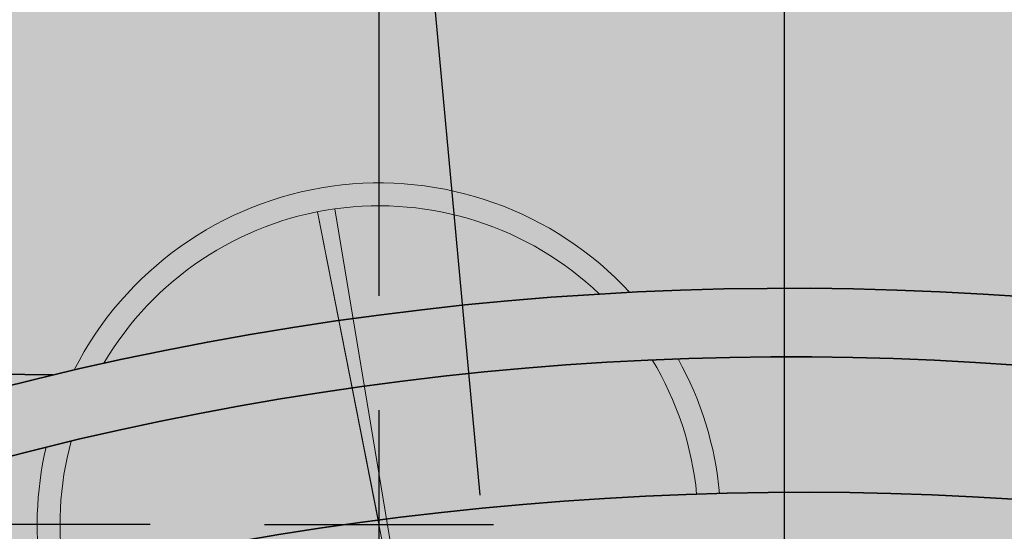
# Model space of a CAD drawing. Units: millimetres. Extents: x 130 to 1021, y 147 to 699.
# Tile 22 of 40: x 399 to 442, y 501 to 523. Entities that reach past the tile are written whole.
import ezdxf

# ---------------------------------------------------------------- set-up
doc = ezdxf.new("R2010")
doc.units = ezdxf.units.MM
doc.header["$MEASUREMENT"] = 0
for name, color, linetype, lineweight in [('A-ANNO-DIMS', 2, 'Continuous', 18), ('A-ELEV', 7, 'Continuous', 35), ('A-ELEV-PATT', 9, 'Continuous', 13), ('A-ELEV-RAIL', 6, 'Continuous', 18)]:
    doc.layers.add(name, color=color, linetype=linetype, lineweight=lineweight)
doc.styles.get("Standard").update_dxf_attribs({"font": 'arial.ttf'})
doc.dimstyles.get("Standard").update_dxf_attribs({"dimtxt": 20, "dimasz": 10, "dimexe": 10, "dimexo": 10, "dimgap": 5, "dimtad": 0, "dimtih": 1, "dimtoh": 1, "dimdec": 0, "dimzin": 0, "dimdsep": 46, "dimtxsty": 'Standard', "dimcen": 5, "dimadec": 0, "dimazin": 0, "dimtfac": 1, "dimtdec": 0, "dimtofl": 0, "dimtmove": 0, "dimatfit": 3, "dimfxl": 1, "dimtolj": 1, "dimtzin": 0, "dimarcsym": 0})

# ---------------------------------------------------------------- blocks, each defined once
blk = doc.blocks.new('*D11')
at = {"layer": 'A-ANNO-DIMS', "color": 0, "lineweight": -2, "transparency": 16777216}
for p, q in [((737.374, 648.699), (737.374, 149.739)), ((299.374, 566.947), (299.374, 149.739)), ((309.374, 159.739), (490.857, 159.739)), ((727.374, 159.739), (545.891, 159.739))]:
    blk.add_line(p, q, dxfattribs=at)
at = {"layer": 'A-ANNO-DIMS', "color": 0, "transparency": 16777216}
for points in [[(309.374, 161.406), (309.374, 158.073), (299.374, 159.739)], [(727.374, 161.406), (727.374, 158.073), (737.374, 159.739)]]:
    blk.add_solid(points, dxfattribs=at)
at = {"layer": 'Defpoints', "color": 0, "transparency": 16777216}
for p in [(737.374, 658.699), (299.374, 576.947), (737.374, 159.739)]:
    blk.add_point(p, dxfattribs=at)
at = {"layer": 'A-ANNO-DIMS', "color": 0, "transparency": 16777216, "insert": (518.374, 159.739), "char_height": 20, "attachment_point": 5}
blk.add_mtext('\\A1;438', dxfattribs=at)
blk = doc.blocks.new('*D12')
at = {"layer": 'A-ANNO-DIMS', "color": 0, "lineweight": -2, "transparency": 16777216}
for p, q in [((477.374, 661.947), (265.074, 661.947)), ((275.074, 651.947), (275.074, 438.205)), ((275.074, 194.039), (275.074, 407.782)), ((357.163, 184.039), (265.074, 184.039))]:
    blk.add_line(p, q, dxfattribs=at)
at = {"layer": 'A-ANNO-DIMS', "color": 0, "transparency": 16777216}
for points in [[(273.407, 651.947), (276.74, 651.947), (275.074, 661.947)], [(273.407, 194.039), (276.74, 194.039), (275.074, 184.039)]]:
    blk.add_solid(points, dxfattribs=at)
at = {"layer": 'Defpoints', "color": 0, "transparency": 16777216}
for p in [(275.074, 661.947), (487.374, 661.947), (367.163, 184.039)]:
    blk.add_point(p, dxfattribs=at)
at = {"layer": 'A-ANNO-DIMS', "color": 0, "transparency": 16777216, "insert": (275.074, 422.993), "char_height": 20, "attachment_point": 5}
blk.add_mtext('\\A1;477.9', dxfattribs=at)
blk = doc.blocks.new('*D15')
at = {"layer": 'A-ANNO-DIMS', "color": 0, "lineweight": -2, "transparency": 16777216}
for p, q in [((327.374, 579.884), (327.374, 696.247)), ((357.941, 411.947), (357.941, 696.247)), ((337.374, 686.247), (347.941, 686.247)), ((357.941, 686.247), (367.941, 686.247))]:
    blk.add_line(p, q, dxfattribs=at)
at = {"layer": 'A-ANNO-DIMS', "color": 0, "transparency": 16777216}
for points in [[(337.374, 687.914), (337.374, 684.581), (327.374, 686.247)], [(347.941, 687.914), (347.941, 684.581), (357.941, 686.247)]]:
    blk.add_solid(points, dxfattribs=at)
at = {"layer": 'Defpoints', "color": 0, "transparency": 16777216}
for p in [(357.941, 686.247), (327.374, 569.884), (357.941, 401.947)]:
    blk.add_point(p, dxfattribs=at)
at = {"layer": 'A-ANNO-DIMS', "color": 0, "transparency": 16777216, "insert": (406.679, 686.247), "char_height": 20, "attachment_point": 5}
blk.add_mtext('\\A1;30.57', dxfattribs=at)
blk = doc.blocks.new('*D16')
at = {"layer": 'A-ANNO-DIMS', "color": 0, "lineweight": -2, "transparency": 16777216}
for p, q in [((357.941, 411.947), (357.941, 696.247)), ((363.922, 579.884), (363.922, 696.247)), ((347.941, 686.247), (337.941, 686.247)), ((373.922, 686.247), (383.922, 686.247))]:
    blk.add_line(p, q, dxfattribs=at)
at = {"layer": 'A-ANNO-DIMS', "color": 0, "transparency": 16777216}
for points in [[(347.941, 687.914), (347.941, 684.581), (357.941, 686.247)], [(373.922, 687.914), (373.922, 684.581), (363.922, 686.247)]]:
    blk.add_solid(points, dxfattribs=at)
at = {"layer": 'Defpoints', "color": 0, "transparency": 16777216}
for p in [(363.922, 686.247), (363.922, 569.884), (357.941, 401.947)]:
    blk.add_point(p, dxfattribs=at)
at = {"layer": 'A-ANNO-DIMS', "color": 0, "transparency": 16777216, "insert": (420.737, 686.247), "char_height": 20, "attachment_point": 5}
blk.add_mtext('\\A1;5.981', dxfattribs=at)
blk = doc.blocks.new('*D17')
at = {"layer": 'A-ANNO-DIMS', "color": 0, "lineweight": -2, "transparency": 16777216}
for p, q in [((363.922, 579.884), (363.922, 696.247)), ((375.85, 490.216), (375.85, 696.247)), ((353.922, 686.247), (343.922, 686.247)), ((385.85, 686.247), (395.85, 686.247))]:
    blk.add_line(p, q, dxfattribs=at)
at = {"layer": 'A-ANNO-DIMS', "color": 0, "transparency": 16777216}
for points in [[(353.922, 687.914), (353.922, 684.581), (363.922, 686.247)], [(385.85, 687.914), (385.85, 684.581), (375.85, 686.247)]]:
    blk.add_solid(points, dxfattribs=at)
at = {"layer": 'Defpoints', "color": 0, "transparency": 16777216}
for p in [(375.85, 686.247), (363.922, 569.884), (375.85, 480.216)]:
    blk.add_point(p, dxfattribs=at)
at = {"layer": 'A-ANNO-DIMS', "color": 0, "transparency": 16777216, "insert": (441.444, 686.247), "char_height": 20, "attachment_point": 5}
blk.add_mtext('\\A1;11.928', dxfattribs=at)
blk = doc.blocks.new('*D18')
at = {"layer": 'A-ANNO-DIMS', "color": 0, "lineweight": -2, "transparency": 16777216}
for p, q in [((375.85, 490.216), (375.85, 696.247)), ((382.374, 388.947), (382.374, 696.247)), ((365.85, 686.247), (355.85, 686.247)), ((392.374, 686.247), (402.374, 686.247))]:
    blk.add_line(p, q, dxfattribs=at)
at = {"layer": 'A-ANNO-DIMS', "color": 0, "transparency": 16777216}
for points in [[(365.85, 687.914), (365.85, 684.581), (375.85, 686.247)], [(392.374, 687.914), (392.374, 684.581), (382.374, 686.247)]]:
    blk.add_solid(points, dxfattribs=at)
at = {"layer": 'Defpoints', "color": 0, "transparency": 16777216}
for p in [(382.374, 686.247), (375.85, 480.216), (382.374, 378.947)]:
    blk.add_point(p, dxfattribs=at)
at = {"layer": 'A-ANNO-DIMS', "color": 0, "transparency": 16777216, "insert": (441.132, 686.247), "char_height": 20, "attachment_point": 5}
blk.add_mtext('\\A1;6.524', dxfattribs=at)
blk = doc.blocks.new('*D19')
at = {"layer": 'A-ANNO-DIMS', "color": 0, "lineweight": -2, "transparency": 16777216}
for p, q in [((382.374, 388.947), (382.374, 696.247)), ((414.652, 510.881), (414.652, 696.247)), ((392.374, 686.247), (404.652, 686.247)), ((414.652, 686.247), (424.652, 686.247))]:
    blk.add_line(p, q, dxfattribs=at)
at = {"layer": 'A-ANNO-DIMS', "color": 0, "transparency": 16777216}
for points in [[(392.374, 687.914), (392.374, 684.581), (382.374, 686.247)], [(404.652, 687.914), (404.652, 684.581), (414.652, 686.247)]]:
    blk.add_solid(points, dxfattribs=at)
at = {"layer": 'Defpoints', "color": 0, "transparency": 16777216}
for p in [(414.652, 686.247), (414.652, 500.881), (382.374, 378.947)]:
    blk.add_point(p, dxfattribs=at)
at = {"layer": 'A-ANNO-DIMS', "color": 0, "transparency": 16777216, "insert": (463.411, 686.247), "char_height": 20, "attachment_point": 5}
blk.add_mtext('\\A1;32.28', dxfattribs=at)
blk = doc.blocks.new('*D20')
at = {"layer": 'A-ANNO-DIMS', "color": 0, "lineweight": -2, "transparency": 16777216}
for p, q in [((414.652, 510.881), (414.652, 696.247)), ((432.374, 388.947), (432.374, 696.247)), ((404.652, 686.247), (394.652, 686.247)), ((442.374, 686.247), (452.374, 686.247))]:
    blk.add_line(p, q, dxfattribs=at)
at = {"layer": 'A-ANNO-DIMS', "color": 0, "transparency": 16777216}
for points in [[(404.652, 687.914), (404.652, 684.581), (414.652, 686.247)], [(442.374, 687.914), (442.374, 684.581), (432.374, 686.247)]]:
    blk.add_solid(points, dxfattribs=at)
at = {"layer": 'Defpoints', "color": 0, "transparency": 16777216}
for p in [(432.374, 686.247), (414.652, 500.881), (432.374, 378.947)]:
    blk.add_point(p, dxfattribs=at)
at = {"layer": 'A-ANNO-DIMS', "color": 0, "transparency": 16777216, "insert": (490.075, 686.247), "char_height": 20, "attachment_point": 5}
blk.add_mtext('\\A1;17.72', dxfattribs=at)
blk = doc.blocks.new('*D21')
at = {"layer": 'A-ANNO-DIMS', "color": 0, "lineweight": -2, "transparency": 16777216}
for p, q in [((432.374, 388.947), (432.374, 696.247)), ((447.374, 656.947), (447.374, 696.247)), ((422.374, 686.247), (412.374, 686.247)), ((457.374, 686.247), (467.374, 686.247))]:
    blk.add_line(p, q, dxfattribs=at)
at = {"layer": 'A-ANNO-DIMS', "color": 0, "transparency": 16777216}
for points in [[(422.374, 687.914), (422.374, 684.581), (432.374, 686.247)], [(457.374, 687.914), (457.374, 684.581), (447.374, 686.247)]]:
    blk.add_solid(points, dxfattribs=at)
at = {"layer": 'Defpoints', "color": 0, "transparency": 16777216}
for p in [(447.374, 686.247), (447.374, 646.947), (432.374, 378.947)]:
    blk.add_point(p, dxfattribs=at)
at = {"layer": 'A-ANNO-DIMS', "color": 0, "transparency": 16777216, "insert": (485.832, 686.247), "char_height": 20, "attachment_point": 5}
blk.add_mtext('\\A1;15', dxfattribs=at)
blk = doc.blocks.new('*D22')
at = {"layer": 'A-ANNO-DIMS', "color": 0, "lineweight": -2, "transparency": 16777216}
for p, q in [((447.374, 656.947), (447.374, 696.247)), ((466.767, 403.947), (466.767, 696.247)), ((437.374, 686.247), (427.374, 686.247)), ((476.767, 686.247), (486.767, 686.247))]:
    blk.add_line(p, q, dxfattribs=at)
at = {"layer": 'A-ANNO-DIMS', "color": 0, "transparency": 16777216}
for points in [[(437.374, 687.914), (437.374, 684.581), (447.374, 686.247)], [(476.767, 687.914), (476.767, 684.581), (466.767, 686.247)]]:
    blk.add_solid(points, dxfattribs=at)
at = {"layer": 'Defpoints', "color": 0, "transparency": 16777216}
for p in [(466.767, 686.247), (447.374, 646.947), (466.767, 393.947)]:
    blk.add_point(p, dxfattribs=at)
at = {"layer": 'A-ANNO-DIMS', "color": 0, "transparency": 16777216, "insert": (532.34, 686.247), "char_height": 20, "attachment_point": 5}
blk.add_mtext('\\A1;19.393', dxfattribs=at)
blk = doc.blocks.new('*D43')
at = {"layer": 'A-ANNO-DIMS', "color": 0, "lineweight": -2, "transparency": 16777216}
for p, q in [((275.074, 510.881), (275.074, 520.881)), ((275.074, 520.881), (285.074, 520.881)), ((404.652, 500.881), (265.074, 500.881)), ((317.374, 480.95), (265.074, 480.95)), ((275.074, 470.95), (275.074, 460.95))]:
    blk.add_line(p, q, dxfattribs=at)
at = {"layer": 'A-ANNO-DIMS', "color": 0, "transparency": 16777216}
for points in [[(273.407, 510.881), (276.74, 510.881), (275.074, 500.881)], [(273.407, 470.95), (276.74, 470.95), (275.074, 480.95)]]:
    blk.add_solid(points, dxfattribs=at)
at = {"layer": 'Defpoints', "color": 0, "transparency": 16777216}
for p in [(275.074, 500.881), (414.652, 500.881), (327.374, 480.95)]:
    blk.add_point(p, dxfattribs=at)
at = {"layer": 'A-ANNO-DIMS', "color": 0, "transparency": 16777216, "insert": (322.877, 520.881), "char_height": 20, "attachment_point": 5}
blk.add_mtext('\\A1;19.93', dxfattribs=at)
blk = doc.blocks.new('*D44')
at = {"layer": 'A-ANNO-DIMS', "color": 0, "lineweight": -2, "transparency": 16777216}
for p, q in [((317.374, 569.884), (265.074, 569.884)), ((275.074, 559.884), (275.074, 550.594)), ((275.074, 510.881), (275.074, 520.171)), ((404.652, 500.881), (265.074, 500.881))]:
    blk.add_line(p, q, dxfattribs=at)
at = {"layer": 'A-ANNO-DIMS', "color": 0, "transparency": 16777216}
for points in [[(273.407, 559.884), (276.74, 559.884), (275.074, 569.884)], [(273.407, 510.881), (276.74, 510.881), (275.074, 500.881)]]:
    blk.add_solid(points, dxfattribs=at)
at = {"layer": 'Defpoints', "color": 0, "transparency": 16777216}
for p in [(275.074, 569.884), (327.374, 569.884), (414.652, 500.881)]:
    blk.add_point(p, dxfattribs=at)
at = {"layer": 'A-ANNO-DIMS', "color": 0, "transparency": 16777216, "insert": (275.074, 535.383), "char_height": 20, "attachment_point": 5}
blk.add_mtext('\\A1;69', dxfattribs=at)
blk = doc.blocks.new('*D62')
at = {"layer": 'A-ANNO-DIMS', "color": 0, "lineweight": -2, "transparency": 16777216}
for p, q in [((414.652, 495.881), (414.652, 505.881)), ((379.725, 501.926), (389.721, 501.627)), ((409.652, 500.881), (419.652, 500.881))]:
    blk.add_line(p, q, dxfattribs=at)
at = {"layer": 'A-ANNO-DIMS', "color": 0, "transparency": 16777216}
blk.add_solid([(389.771, 503.293), (389.671, 499.961), (399.716, 501.328)], dxfattribs=at)
at = {"layer": 'Defpoints', "color": 0, "transparency": 16777216}
for p in [(399.716, 501.328), (429.589, 500.434)]:
    blk.add_point(p, dxfattribs=at)
at = {"layer": 'A-ANNO-DIMS', "color": 0, "transparency": 16777216, "insert": (322.338, 501.926), "char_height": 20, "attachment_point": 5}
blk.add_mtext('\\A1;∅29.886', dxfattribs=at)
blk = doc.blocks.new('*D63')
at = {"layer": 'A-ANNO-DIMS', "color": 0, "lineweight": -2, "transparency": 16777216}
for p, q in [((414.652, 495.881), (414.652, 505.881)), ((380.753, 502.59), (390.74, 502.086)), ((409.652, 500.881), (419.652, 500.881))]:
    blk.add_line(p, q, dxfattribs=at)
at = {"layer": 'A-ANNO-DIMS', "color": 0, "transparency": 16777216}
blk.add_solid([(390.824, 503.751), (390.656, 500.422), (400.727, 501.583)], dxfattribs=at)
at = {"layer": 'Defpoints', "color": 0, "transparency": 16777216}
for p in [(400.727, 501.583), (428.578, 500.179)]:
    blk.add_point(p, dxfattribs=at)
at = {"layer": 'A-ANNO-DIMS', "color": 0, "transparency": 16777216, "insert": (323.365, 502.59), "char_height": 20, "attachment_point": 5}
blk.add_mtext('\\A1;∅27.886', dxfattribs=at)
blk = doc.blocks.new('*D65')
at = {"layer": 'A-ANNO-DIMS', "color": 0, "lineweight": -2, "transparency": 16777216}
for p, q in [((495.463, 509.127), (472.508, 423.108)), ((505.463, 509.127), (495.463, 509.127)), ((427.374, 248.979), (427.374, 258.979)), ((422.374, 253.979), (432.374, 253.979))]:
    blk.add_line(p, q, dxfattribs=at)
at = {"layer": 'A-ANNO-DIMS', "color": 0, "transparency": 16777216}
blk.add_solid([(470.898, 423.538), (474.118, 422.679), (469.93, 413.447)], dxfattribs=at)
at = {"layer": 'Defpoints', "color": 0, "transparency": 16777216}
for p in [(469.93, 413.447), (427.374, 253.979)]:
    blk.add_point(p, dxfattribs=at)
at = {"layer": 'A-ANNO-DIMS', "color": 0, "transparency": 16777216, "insert": (561.623, 509.127), "char_height": 20, "attachment_point": 5}
blk.add_mtext('\\A1;R165.05', dxfattribs=at)
blk = doc.blocks.new('*D66')
at = {"layer": 'A-ANNO-DIMS', "color": 0, "lineweight": -2, "transparency": 16777216}
for p, q in [((341.579, 557.194), (351.579, 557.194)), ((351.579, 557.194), (376.947, 478.135)), ((427.374, 315.978), (427.374, 325.978)), ((422.374, 320.978), (432.374, 320.978))]:
    blk.add_line(p, q, dxfattribs=at)
at = {"layer": 'A-ANNO-DIMS', "color": 0, "transparency": 16777216}
blk.add_solid([(378.534, 478.644), (375.36, 477.626), (380.002, 468.613)], dxfattribs=at)
at = {"layer": 'Defpoints', "color": 0, "transparency": 16777216}
for p in [(380.002, 468.613), (427.374, 320.978)]:
    blk.add_point(p, dxfattribs=at)
at = {"layer": 'A-ANNO-DIMS', "color": 0, "transparency": 16777216, "insert": (263.53, 557.194), "char_height": 20, "attachment_point": 5}
blk.add_mtext('\\A1;4X R155.05', dxfattribs=at)
blk = doc.blocks.new('*D67')
at = {"layer": 'A-ANNO-DIMS', "color": 0, "lineweight": -2, "transparency": 16777216}
for p, q in [((479.756, 492.431), (462.144, 412.223)), ((489.756, 492.431), (479.756, 492.431)), ((427.07, 247.496), (427.07, 257.496)), ((422.07, 252.496), (432.07, 252.496))]:
    blk.add_line(p, q, dxfattribs=at)
at = {"layer": 'A-ANNO-DIMS', "color": 0, "transparency": 16777216}
blk.add_solid([(460.516, 412.58), (463.772, 411.865), (459.999, 402.455)], dxfattribs=at)
at = {"layer": 'Defpoints', "color": 0, "transparency": 16777216}
for p in [(459.999, 402.455), (427.07, 252.496)]:
    blk.add_point(p, dxfattribs=at)
at = {"layer": 'A-ANNO-DIMS', "color": 0, "transparency": 16777216, "insert": (545.841, 492.431), "char_height": 20, "attachment_point": 5}
blk.add_mtext('\\A1;R153.53', dxfattribs=at)
blk = doc.blocks.new('*D68')
at = {"layer": 'A-ANNO-DIMS', "color": 0, "lineweight": -2, "transparency": 16777216}
for p, q in [((361.841, 579.756), (371.841, 579.756)), ((371.841, 579.756), (392.167, 506.693)), ((433.191, 354.23), (433.191, 364.23)), ((428.191, 359.23), (438.191, 359.23))]:
    blk.add_line(p, q, dxfattribs=at)
at = {"layer": 'A-ANNO-DIMS', "color": 0, "transparency": 16777216}
blk.add_solid([(393.773, 507.14), (390.561, 506.246), (394.847, 497.059)], dxfattribs=at)
at = {"layer": 'Defpoints', "color": 0, "transparency": 16777216}
for p in [(394.847, 497.059), (433.191, 359.23)]:
    blk.add_point(p, dxfattribs=at)
at = {"layer": 'A-ANNO-DIMS', "color": 0, "transparency": 16777216, "insert": (305.764, 579.756), "char_height": 20, "attachment_point": 5}
blk.add_mtext('\\A1;R143.06', dxfattribs=at)
blk = doc.blocks.new('*D69')
at = {"layer": 'A-ANNO-DIMS', "color": 0, "lineweight": -2, "transparency": 16777216}
for p, q in [((507.746, 572.261), (483.091, 501.813)), ((517.746, 572.261), (507.746, 572.261)), ((433.191, 354.23), (433.191, 364.23)), ((428.191, 359.23), (438.191, 359.23))]:
    blk.add_line(p, q, dxfattribs=at)
at = {"layer": 'A-ANNO-DIMS', "color": 0, "transparency": 16777216}
blk.add_solid([(481.518, 502.363), (484.664, 501.262), (479.788, 492.374)], dxfattribs=at)
at = {"layer": 'Defpoints', "color": 0, "transparency": 16777216}
for p in [(479.788, 492.374), (433.191, 359.23)]:
    blk.add_point(p, dxfattribs=at)
at = {"layer": 'A-ANNO-DIMS', "color": 0, "transparency": 16777216, "insert": (573.824, 572.261), "char_height": 20, "attachment_point": 5}
blk.add_mtext('\\A1;R141.06', dxfattribs=at)
blk = doc.blocks.new('*D70')
at = {"layer": 'A-ANNO-DIMS', "color": 0, "lineweight": -2, "transparency": 16777216}
for p, q in [((370.141, 588.4), (380.141, 588.4)), ((380.141, 588.4), (397.473, 517.008)), ((432.65, 367.109), (432.65, 377.109)), ((427.65, 372.109), (437.65, 372.109))]:
    blk.add_line(p, q, dxfattribs=at)
at = {"layer": 'A-ANNO-DIMS', "color": 0, "transparency": 16777216}
blk.add_solid([(399.093, 517.402), (395.854, 516.615), (399.832, 507.291)], dxfattribs=at)
at = {"layer": 'Defpoints', "color": 0, "transparency": 16777216}
for p in [(399.832, 507.291), (432.65, 372.109)]:
    blk.add_point(p, dxfattribs=at)
at = {"layer": 'A-ANNO-DIMS', "color": 0, "transparency": 16777216, "insert": (323.757, 588.4), "char_height": 20, "attachment_point": 5}
blk.add_mtext('\\A1;R139.1', dxfattribs=at)
blk = doc.blocks.new('*D71')
at = {"layer": 'A-ANNO-DIMS', "color": 0, "lineweight": -2, "transparency": 16777216}
for p, q in [((492.108, 581.609), (472.542, 512.666)), ((502.108, 581.609), (492.108, 581.609)), ((432.65, 367.109), (432.65, 377.109)), ((427.65, 372.109), (437.65, 372.109))]:
    blk.add_line(p, q, dxfattribs=at)
at = {"layer": 'A-ANNO-DIMS', "color": 0, "transparency": 16777216}
blk.add_solid([(470.938, 513.121), (474.145, 512.211), (469.812, 503.046)], dxfattribs=at)
at = {"layer": 'Defpoints', "color": 0, "transparency": 16777216}
for p in [(469.812, 503.046), (432.65, 372.109)]:
    blk.add_point(p, dxfattribs=at)
at = {"layer": 'A-ANNO-DIMS', "color": 0, "transparency": 16777216, "insert": (548.493, 581.609), "char_height": 20, "attachment_point": 5}
blk.add_mtext('\\A1;R136.1', dxfattribs=at)
blk = doc.blocks.new('*D72')
at = {"layer": 'A-ANNO-DIMS', "color": 0, "lineweight": -2, "transparency": 16777216}
for p, q in [((460.658, 573.64), (451.279, 503.49)), ((470.658, 573.64), (460.658, 573.64)), ((432.115, 355.142), (432.115, 365.142)), ((427.115, 360.142), (437.115, 360.142))]:
    blk.add_line(p, q, dxfattribs=at)
at = {"layer": 'A-ANNO-DIMS', "color": 0, "transparency": 16777216}
blk.add_solid([(449.628, 503.711), (452.931, 503.27), (449.954, 493.579)], dxfattribs=at)
at = {"layer": 'Defpoints', "color": 0, "transparency": 16777216}
for p in [(449.954, 493.579), (432.115, 360.142)]:
    blk.add_point(p, dxfattribs=at)
at = {"layer": 'A-ANNO-DIMS', "color": 0, "transparency": 16777216, "insert": (526.64, 573.64), "char_height": 20, "attachment_point": 5}
blk.add_mtext('\\A1;R134.62', dxfattribs=at)
blk = doc.blocks.new('*D73')
at = {"layer": 'A-ANNO-DIMS', "color": 0, "lineweight": -2, "transparency": 16777216}
for p, q in [((402.678, 571.448), (412.678, 571.448)), ((412.678, 571.448), (419.051, 502.166)), ((432.115, 355.142), (432.115, 365.142)), ((427.115, 360.142), (437.115, 360.142))]:
    blk.add_line(p, q, dxfattribs=at)
at = {"layer": 'A-ANNO-DIMS', "color": 0, "transparency": 16777216}
blk.add_solid([(420.711, 502.319), (417.391, 502.014), (419.967, 492.208)], dxfattribs=at)
at = {"layer": 'Defpoints', "color": 0, "transparency": 16777216}
for p in [(419.967, 492.208), (432.115, 360.142)]:
    blk.add_point(p, dxfattribs=at)
at = {"layer": 'A-ANNO-DIMS', "color": 0, "transparency": 16777216, "insert": (346.696, 571.448), "char_height": 20, "attachment_point": 5}
blk.add_mtext('\\A1;R132.62', dxfattribs=at)

msp = doc.modelspace()

# ---------------------------------------------------------------- hatches: boundary and pattern name
at = {"layer": 'A-ELEV-PATT'}
h = msp.add_hatch(color=256, dxfattribs=at)
h.dxf.hatch_style = 1
h.paths.add_polyline_path([(737.3738, 658.6988, 0.0135961), (632.4019, 661.9473), (607.3738, 661.9473), (487.3738, 661.9473), (487.3738, 649.9473), (607.3738, 649.9473), (632.3794, 649.9473, -0.0136841), (737.3738, 646.6784)])
h.paths.add_polyline_path([(732.3738, 643.9599, 0.0130529), (632.3738, 646.9473), (607.3738, 646.9473), (487.3738, 646.9473), (487.3738, 596.9473), (632.3738, 596.9473, -0.0130529), (732.3738, 593.9599)])
h.paths.add_polyline_path([(737.3738, 593.6732, 0.0137063), (632.3738, 596.9473), (487.3738, 596.9473), (487.3738, 586.9473), (632.355, 586.9473, -0.0137808), (737.3738, 583.6559)])
h.paths.add_polyline_path([(447.3738, 646.9473), (307.3738, 646.9473), (302.3738, 646.9473), (302.3738, 634.9473), (447.3738, 634.9473)])
h.paths.add_polyline_path([(447.3738, 631.9473), (307.3738, 631.9473), (307.3738, 586.9473), (447.3738, 586.9473)])
h.paths.add_polyline_path([(447.3738, 586.9473), (307.3738, 586.9473), (302.3738, 586.9473), (302.3738, 576.9473), (447.3738, 576.9473)])
h.paths.add_polyline_path([(447.3738, 573.9473), (367.3738, 573.9473), (367.3738, 539.9473), (447.3738, 539.9473)])
h.paths.add_polyline_path([(447.3738, 537.9473), (367.3738, 537.9473), (367.3738, 507.9473), (400.392, 507.4253, -0.001728), (401.3281, 507.6451, -0.5220025), (425.6117, 511.0391, -0.0391849), (447.3738, 510.4359), (447.3738, 510.7883)])
h.paths.add_polyline_path([(394.7238, 505.9473), (367.3738, 505.9473), (367.3738, 476.9473, -0.0146512), (375.8501, 480.2159), (376.1506, 499.2266, -0.0355419)])
h.paths.add_polyline_path([(632.3738, 583.9473), (552.3738, 583.9473), (552.3738, 550.9473), (632.3738, 550.9473)])
h.paths.add_polyline_path([(632.3738, 548.9473), (552.3738, 548.9473), (552.3738, 515.9473), (632.3738, 515.9473)])
h.paths.add_polyline_path([(632.3738, 513.9473), (552.3738, 513.9473), (552.3738, 476.9473), (632.3738, 476.9473)])
h.paths.add_polyline_path([(737.3738, 473.6903, 0.0136326), (632.3926, 476.9473), (552.3738, 476.9473), (487.3738, 476.9473), (487.3738, 466.9473), (632.3738, 466.9473, -0.0137063), (737.3738, 463.6732)])
h.paths.add_polyline_path([(732.3738, 460.9552, 0.0130741), (632.3681, 463.9473), (487.3738, 463.9473), (487.3738, 407.735, -0.0032286), (489.3544, 406.9473), (632.3926, 406.9473, -0.0129826), (732.3738, 403.9755)])
h.paths.add_polyline_path([(487.3738, 463.9473, 0.20133), (367.3738, 463.9473), (367.3738, 407.735, -0.1882031), (487.3738, 407.735)])
h.paths.add_polyline_path([(367.3738, 476.9473), (367.3738, 466.9473, -0.2013309), (487.3738, 466.9473), (487.3738, 476.9473, 0.20133)])
h.paths.add_polyline_path([(367.3738, 463.9473), (307.3738, 463.9473), (307.3738, 401.9473), (357.9413, 401.9473), (367.3738, 407.735)])
h.paths.add_polyline_path([(367.3738, 476.9473), (302.3738, 476.9473), (302.3738, 466.9473), (367.3738, 466.9473)])
h.paths.add_polyline_path([(632.8184, 366.9453), (552.3738, 366.9453), (552.3738, 393.9473), (632.8184, 393.9473)])
h.paths.add_polyline_path([(632.8184, 357.2114), (632.8184, 363.9453), (552.3738, 363.9453), (552.3738, 357.2114), (552.3738, 336.9453), (632.8184, 336.9453)])
h.paths.add_polyline_path([(632.8184, 333.9453), (552.3738, 333.9453), (552.3738, 306.9453), (632.8184, 306.9453)])
h.paths.add_polyline_path([(632.8184, 303.9453), (552.3738, 303.9453), (552.3738, 273.9473), (632.355, 273.9473, 0.0000608), (632.8184, 273.9491)])
h.paths.add_polyline_path([(737.3738, 403.6903, 0.0136326), (632.3926, 406.9473), (489.3544, 406.9473, 0.1915481), (367.3738, 407.735), (367.3738, 396.9473, -0.2013309), (487.3738, 396.9473), (632.3738, 396.9473, -0.0137063), (737.3738, 393.6732)])
h.paths.add_polyline_path([(357.9413, 401.9473), (307.3738, 401.9473), (307.3738, 391.9473), (357.9413, 391.9473)])
h.paths.add_polyline_path([(357.9413, 357.2114), (357.9413, 388.9473), (307.3738, 388.9473), (307.3738, 357.2114), (307.3738, 273.9473), (357.9413, 273.9473)])
h.paths.add_polyline_path([(732.3738, 263.93, -0.0130317), (632.3794, 260.9473), (466.7667, 260.9473), (466.7667, 240.9473), (469.8406, 236.978), (469.8406, 221.978), (472.9145, 218.0087), (472.9145, 213.9473), (607.3738, 213.9473), (732.3738, 213.9473)])
h.paths.add_polyline_path([(732.3738, 290.889), (722.479, 290.889), (722.479, 301.889), (732.3738, 301.889), (732.3738, 305.889), (722.479, 305.889), (722.479, 316.889), (732.3738, 316.889), (732.3738, 320.889), (722.479, 320.889), (722.479, 331.889), (732.3738, 331.889), (732.3738, 335.889), (722.479, 335.889), (722.479, 346.889), (732.3738, 346.889), (732.3738, 350.889), (722.479, 350.889), (722.479, 361.889), (732.3738, 361.889), (732.3738, 365.889), (722.479, 365.889), (722.479, 376.889), (732.3738, 376.889), (732.3738, 380.889), (722.479, 380.889), (722.479, 391.4848, 0.0005233), (718.479, 391.6843), (718.479, 380.889), (707.479, 380.889), (707.479, 392.1896, 0.0005231), (703.479, 392.3576), (703.479, 380.889), (692.479, 380.889), (692.479, 392.7765, 0.0005229), (688.479, 392.9131), (688.479, 380.889), (677.479, 380.889), (677.479, 393.2456, 0.0005228), (673.479, 393.3508), (673.479, 380.889), (662.479, 380.889), (662.479, 393.597, 0.0005227), (658.479, 393.6709), (658.479, 380.889), (647.479, 380.889), (647.479, 393.8308, 0.0005226), (643.479, 393.8732), (643.479, 380.889), (632.8184, 380.889), (632.8184, 376.889), (643.479, 376.889), (643.479, 365.889), (632.8184, 365.889), (632.8184, 361.889), (643.479, 361.889), (643.479, 350.889), (632.8184, 350.889), (632.8184, 346.889), (643.479, 346.889), (643.479, 335.889), (632.8184, 335.889), (632.8184, 331.889), (643.479, 331.889), (643.479, 320.889), (632.8184, 320.889), (632.8184, 316.889), (643.479, 316.889), (643.479, 305.889), (632.8184, 305.889), (632.8184, 301.889), (643.479, 301.889), (643.479, 290.889), (632.8184, 290.889), (632.8184, 286.889), (643.479, 286.889), (643.479, 274.0217, 0.0005246), (647.479, 274.0643), (647.479, 286.889), (658.479, 286.889), (658.479, 274.2248, 0.0005246), (662.479, 274.2989), (662.479, 286.889), (673.479, 286.889), (673.479, 274.546, 0.0005247), (677.479, 274.6516), (677.479, 286.889), (688.479, 286.889), (688.479, 274.9853, 0.0005248), (692.479, 275.1224), (692.479, 286.889), (703.479, 286.889), (703.479, 275.5429, 0.000525), (707.479, 275.7115), (707.479, 286.889), (718.479, 286.889), (718.479, 276.2187, 0.0005252), (722.479, 276.4189), (722.479, 286.889), (732.3738, 286.889)])
h.paths.add_polyline_path([(718.479, 290.889), (707.479, 290.889), (707.479, 301.889), (718.479, 301.889)], flags=16)
h.paths.add_polyline_path([(703.479, 290.889), (692.479, 290.889), (692.479, 301.889), (703.479, 301.889)], flags=16)
h.paths.add_polyline_path([(718.479, 305.889), (707.479, 305.889), (707.479, 316.889), (718.479, 316.889)], flags=16)
h.paths.add_polyline_path([(703.479, 305.889), (692.479, 305.889), (692.479, 316.889), (703.479, 316.889)], flags=16)
h.paths.add_polyline_path([(688.479, 290.889), (677.479, 290.889), (677.479, 301.889), (688.479, 301.889)], flags=16)
h.paths.add_polyline_path([(718.479, 320.889), (707.479, 320.889), (707.479, 331.889), (718.479, 331.889)], flags=16)
h.paths.add_polyline_path([(688.479, 305.889), (677.479, 305.889), (677.479, 316.889), (688.479, 316.889)], flags=16)
h.paths.add_polyline_path([(703.479, 320.889), (692.479, 320.889), (692.479, 331.889), (703.479, 331.889)], flags=16)
h.paths.add_polyline_path([(688.479, 320.889), (677.479, 320.889), (677.479, 331.889), (688.479, 331.889)], flags=16)
h.paths.add_polyline_path([(673.479, 290.889), (662.479, 290.889), (662.479, 301.889), (673.479, 301.889)], flags=16)
h.paths.add_polyline_path([(718.479, 335.889), (707.479, 335.889), (707.479, 346.889), (718.479, 346.889)], flags=16)
h.paths.add_polyline_path([(673.479, 305.889), (662.479, 305.889), (662.479, 316.889), (673.479, 316.889)], flags=16)
h.paths.add_polyline_path([(703.479, 335.889), (692.479, 335.889), (692.479, 346.889), (703.479, 346.889)], flags=16)
h.paths.add_polyline_path([(673.479, 320.889), (662.479, 320.889), (662.479, 331.889), (673.479, 331.889)], flags=16)
h.paths.add_polyline_path([(688.479, 335.889), (677.479, 335.889), (677.479, 346.889), (688.479, 346.889)], flags=16)
h.paths.add_polyline_path([(658.479, 290.889), (647.479, 290.889), (647.479, 301.889), (658.479, 301.889)], flags=16)
h.paths.add_polyline_path([(718.479, 350.889), (707.479, 350.889), (707.479, 361.889), (718.479, 361.889)], flags=16)
h.paths.add_polyline_path([(658.479, 305.889), (647.479, 305.889), (647.479, 316.889), (658.479, 316.889)], flags=16)
h.paths.add_polyline_path([(703.479, 350.889), (692.479, 350.889), (692.479, 361.889), (703.479, 361.889)], flags=16)
h.paths.add_polyline_path([(673.479, 335.889), (662.479, 335.889), (662.479, 346.889), (673.479, 346.889)], flags=16)
h.paths.add_polyline_path([(658.479, 320.889), (647.479, 320.889), (647.479, 331.889), (658.479, 331.889)], flags=16)
h.paths.add_polyline_path([(688.479, 350.889), (677.479, 350.889), (677.479, 361.889), (688.479, 361.889)], flags=16)
h.paths.add_polyline_path([(718.479, 365.889), (707.479, 365.889), (707.479, 376.889), (718.479, 376.889)], flags=16)
h.paths.add_polyline_path([(658.479, 335.889), (647.479, 335.889), (647.479, 346.889), (658.479, 346.889)], flags=16)
h.paths.add_polyline_path([(673.479, 350.889), (662.479, 350.889), (662.479, 361.889), (673.479, 361.889)], flags=16)
h.paths.add_polyline_path([(703.479, 365.889), (692.479, 365.889), (692.479, 376.889), (703.479, 376.889)], flags=16)
h.paths.add_polyline_path([(688.479, 365.889), (677.479, 365.889), (677.479, 376.889), (688.479, 376.889)], flags=16)
h.paths.add_polyline_path([(658.479, 350.889), (647.479, 350.889), (647.479, 361.889), (658.479, 361.889)], flags=16)
h.paths.add_polyline_path([(673.479, 365.889), (662.479, 365.889), (662.479, 376.889), (673.479, 376.889)], flags=16)
h.paths.add_polyline_path([(658.479, 365.889), (647.479, 365.889), (647.479, 376.889), (658.479, 376.889)], flags=16)
h.paths.add_polyline_path([(732.3738, 503.9786), (722.3392, 503.9786), (722.3392, 514.9786), (732.3738, 514.9786), (732.3738, 518.9786), (722.3392, 518.9786), (722.3392, 529.9786), (732.3738, 529.9786), (732.3738, 533.9786), (722.3392, 533.9786), (722.3392, 544.9786), (732.3738, 544.9786), (732.3738, 546.9473), (732.3738, 548.9786), (722.3392, 548.9786), (722.3392, 559.9786), (732.3738, 559.9786), (732.3738, 563.9786), (722.3392, 563.9786), (722.3392, 574.9786), (732.3738, 574.9786), (732.3738, 578.9786), (722.3392, 578.9786), (722.3392, 581.4789, 0.000526), (718.3392, 581.6791), (718.3392, 578.9786), (707.3392, 578.9786), (707.3392, 582.1863, 0.0005258), (703.3392, 582.355), (703.3392, 578.9786), (692.3392, 578.9786), (692.3392, 582.7752, 0.0005257), (688.3392, 582.9123), (688.3392, 578.9786), (677.3392, 578.9786), (677.3392, 583.2457, 0.0005255), (673.3392, 583.3512), (673.3392, 578.9786), (662.3392, 578.9786), (662.3392, 583.5978, 0.0005254), (658.3392, 583.6718), (658.3392, 578.9786), (647.3392, 578.9786), (647.3392, 583.8317, 0.0005254), (643.3392, 583.8741), (643.3392, 578.9786), (632.3738, 578.9786), (632.3738, 574.9786), (643.3392, 574.9786), (643.3392, 563.9786), (632.3738, 563.9786), (632.3738, 559.9786), (643.3392, 559.9786), (643.3392, 548.9786), (632.3738, 548.9786), (632.3738, 544.9786), (643.3392, 544.9786), (643.3392, 533.9786), (632.3738, 533.9786), (632.3738, 529.9786), (643.3392, 529.9786), (643.3392, 518.9786), (632.3738, 518.9786), (632.3738, 515.9473), (632.3738, 514.9786), (643.3392, 514.9786), (643.3392, 503.9786), (632.3738, 503.9786), (632.3738, 499.9786), (643.3392, 499.9786), (643.3392, 488.9786), (632.3738, 488.9786), (632.3738, 484.9786), (643.3392, 484.9786), (643.3392, 476.8751, -0.0005191), (647.3392, 476.8332), (647.3392, 484.9786), (658.3392, 484.9786), (658.3392, 476.6752, -0.0005192), (662.3392, 476.6022), (662.3392, 484.9786), (673.3392, 484.9786), (673.3392, 476.3585, -0.0005193), (677.3392, 476.2543), (677.3392, 484.9786), (688.3392, 484.9786), (688.3392, 475.9248, -0.0005194), (692.3392, 475.7894), (692.3392, 484.9786), (703.3392, 484.9786), (703.3392, 475.3741, -0.0005195), (707.3392, 475.2075), (707.3392, 484.9786), (718.3392, 484.9786), (718.3392, 474.7064, -0.0005197), (722.3392, 474.5086), (722.3392, 484.9786), (732.3738, 484.9786), (732.3738, 488.9786), (722.3392, 488.9786), (722.3392, 499.9786), (732.3738, 499.9786)])
h.paths.add_polyline_path([(718.3392, 503.9786), (707.3392, 503.9786), (707.3392, 514.9786), (718.3392, 514.9786)], flags=16)
h.paths.add_polyline_path([(718.3392, 499.9786), (718.3392, 488.9786), (707.3392, 488.9786), (707.3392, 499.9786)], flags=16)
h.paths.add_polyline_path([(718.3392, 518.9786), (707.3392, 518.9786), (707.3392, 529.9786), (718.3392, 529.9786)], flags=16)
h.paths.add_polyline_path([(703.3392, 503.9786), (692.3392, 503.9786), (692.3392, 514.9786), (703.3392, 514.9786)], flags=16)
h.paths.add_polyline_path([(703.3392, 499.9786), (703.3392, 488.9786), (692.3392, 488.9786), (692.3392, 499.9786)], flags=16)
h.paths.add_polyline_path([(703.3392, 518.9786), (692.3392, 518.9786), (692.3392, 529.9786), (703.3392, 529.9786)], flags=16)
h.paths.add_polyline_path([(718.3392, 533.9786), (707.3392, 533.9786), (707.3392, 544.9786), (718.3392, 544.9786)], flags=16)
h.paths.add_polyline_path([(688.3392, 503.9786), (677.3392, 503.9786), (677.3392, 514.9786), (688.3392, 514.9786)], flags=16)
h.paths.add_polyline_path([(688.3392, 499.9786), (688.3392, 488.9786), (677.3392, 488.9786), (677.3392, 499.9786)], flags=16)
h.paths.add_polyline_path([(703.3392, 533.9786), (692.3392, 533.9786), (692.3392, 544.9786), (703.3392, 544.9786)], flags=16)
h.paths.add_polyline_path([(688.3392, 518.9786), (677.3392, 518.9786), (677.3392, 529.9786), (688.3392, 529.9786)], flags=16)
h.paths.add_polyline_path([(688.3392, 533.9786), (677.3392, 533.9786), (677.3392, 544.9786), (688.3392, 544.9786)], flags=16)
h.paths.add_polyline_path([(718.3392, 548.9786), (707.3392, 548.9786), (707.3392, 559.9786), (718.3392, 559.9786)], flags=16)
h.paths.add_polyline_path([(673.3392, 503.9786), (662.3392, 503.9786), (662.3392, 514.9786), (673.3392, 514.9786)], flags=16)
h.paths.add_polyline_path([(673.3392, 499.9786), (673.3392, 488.9786), (662.3392, 488.9786), (662.3392, 499.9786)], flags=16)
h.paths.add_polyline_path([(703.3392, 548.9786), (692.3392, 548.9786), (692.3392, 559.9786), (703.3392, 559.9786)], flags=16)
h.paths.add_polyline_path([(673.3392, 518.9786), (662.3392, 518.9786), (662.3392, 529.9786), (673.3392, 529.9786)], flags=16)
h.paths.add_polyline_path([(688.3392, 548.9786), (677.3392, 548.9786), (677.3392, 559.9786), (688.3392, 559.9786)], flags=16)
h.paths.add_polyline_path([(673.3392, 533.9786), (662.3392, 533.9786), (662.3392, 544.9786), (673.3392, 544.9786)], flags=16)
h.paths.add_polyline_path([(718.3392, 563.9786), (707.3392, 563.9786), (707.3392, 574.9786), (718.3392, 574.9786)], flags=16)
h.paths.add_polyline_path([(658.3392, 503.9786), (647.3392, 503.9786), (647.3392, 514.9786), (658.3392, 514.9786)], flags=16)
h.paths.add_polyline_path([(658.3392, 499.9786), (658.3392, 488.9786), (647.3392, 488.9786), (647.3392, 499.9786)], flags=16)
h.paths.add_polyline_path([(703.3392, 563.9786), (692.3392, 563.9786), (692.3392, 574.9786), (703.3392, 574.9786)], flags=16)
h.paths.add_polyline_path([(658.3392, 518.9786), (647.3392, 518.9786), (647.3392, 529.9786), (658.3392, 529.9786)], flags=16)
h.paths.add_polyline_path([(673.3392, 548.9786), (662.3392, 548.9786), (662.3392, 559.9786), (673.3392, 559.9786)], flags=16)
h.paths.add_polyline_path([(688.3392, 563.9786), (677.3392, 563.9786), (677.3392, 574.9786), (688.3392, 574.9786)], flags=16)
h.paths.add_polyline_path([(658.3392, 533.9786), (647.3392, 533.9786), (647.3392, 544.9786), (658.3392, 544.9786)], flags=16)
h.paths.add_polyline_path([(673.3392, 563.9786), (662.3392, 563.9786), (662.3392, 574.9786), (673.3392, 574.9786)], flags=16)
h.paths.add_polyline_path([(658.3392, 548.9786), (647.3392, 548.9786), (647.3392, 559.9786), (658.3392, 559.9786)], flags=16)
h.paths.add_polyline_path([(658.3392, 563.9786), (647.3392, 563.9786), (647.3392, 574.9786), (658.3392, 574.9786)], flags=16)
h = msp.add_hatch(color=256, dxfattribs=at)
h.dxf.hatch_style = 1
h.paths.add_polyline_path([(447.3738, 537.9473), (447.3738, 539.9473), (367.3738, 539.9473), (367.3738, 537.9473)])
h.paths.add_polyline_path([(394.7238, 505.9473, -0.0105284), (400.392, 507.4253), (367.3738, 507.9473), (367.3738, 505.9473)])
h.paths.add_polyline_path([(547.7773, 546.9473), (547.7773, 548.9473), (502.3738, 548.9473), (502.3738, 546.9473)])
h.paths.add_polyline_path([(632.3738, 548.9473), (632.3738, 550.9473), (552.3738, 550.9473), (552.3738, 548.9473)])
h.paths.add_polyline_path([(632.3738, 513.9473), (632.3738, 515.9473), (552.3738, 515.9473), (552.3738, 513.9473)])
h.paths.add_polyline_path([(544.6354, 360.9453), (544.6354, 363.9453), (486.7667, 363.9454), (486.7667, 360.9454)])
h.paths.add_polyline_path([(632.8184, 363.9453), (632.8184, 366.9453), (552.3738, 366.9453), (552.3738, 363.9453)])
h.paths.add_polyline_path([(632.8184, 333.9453), (632.8184, 336.9453), (552.3738, 336.9453), (552.3738, 333.9453)])
h.paths.add_polyline_path([(552.3738, 306.9453), (552.3738, 303.9453), (632.8184, 303.9453), (632.8184, 306.9453)])
h = msp.add_hatch(color=256, dxfattribs=at)
h.paths.add_polyline_path([(424.2813, 510.9653, -0.0023948), (425.6117, 511.0391, 0.5220025), (401.3281, 507.6451, -0.0023948), (402.6278, 507.9389, -0.4837736)])
h.paths.add_polyline_path([(401.1963, 504.533, 0.002075), (400.0983, 504.2673, 0.0996756), (399.9219, 498.3708, -0.0017511), (400.8973, 498.6004, -0.1077432)])
h.paths.add_polyline_path([(401.3652, 496.6558, 0.0017772), (400.3891, 496.4261, 0.0927216), (402.9637, 491.5717, -0.0020893), (404.0631, 491.8108, -0.1004366)])
h.paths.add_polyline_path([(427.7205, 508.128, 0.002075), (426.5918, 508.0824, -0.1121628), (428.5313, 502.2169, -0.0017511), (429.5329, 502.2461, 0.1040877)])
h.paths.add_polyline_path([(429.5819, 500.2467, 0.0017772), (428.5796, 500.2174, -0.1038146), (427.1375, 494.6738, -0.0020893), (428.2619, 494.7107, 0.0960946)])
h.paths.add_polyline_path([(427.1388, 492.6724, 0.0023673), (425.8841, 492.6194, -0.0992667), (421.8309, 488.928, -0.0030044), (423.6933, 488.9834, 0.0850627)])
h.paths.add_polyline_path([(405.7805, 490.125, 0.0023673), (404.5509, 489.8698, 0.061248), (407.5193, 487.7506, -0.0030044), (409.3686, 487.9781, -0.0753981)])
h = msp.add_hatch(color=256, dxfattribs=at)
h.paths.add_polyline_path([(426.5918, 508.0824, 0.047204), (401.1963, 504.533, 0.1077432), (400.8973, 498.6004, -0.0488179), (428.5313, 502.2169, 0.1121628)])
h.paths.add_polyline_path([(424.2813, 510.9653, 0.4837736), (402.6278, 507.9389, -0.0393538)])
h.paths.add_polyline_path([(428.5796, 500.2174, 0.0487581), (401.3652, 496.6558, 0.1004366), (404.0631, 491.8108, -0.0432592), (427.1375, 494.6738, 0.1038146)])
h.paths.add_polyline_path([(425.8841, 492.6194, 0.0382424), (405.7805, 490.125, 0.0753981), (409.3686, 487.9781, -0.0201605), (421.8309, 488.928, 0.0992667)])
h = msp.add_hatch(color=256, dxfattribs=at)
h.paths.add_polyline_path([(375.8501, 480.2159, -0.0051389), (378.8667, 481.244), (378.8725, 481.6093, -0.2220519), (491.1023, 478.9257), (491.1023, 476.9473), (494.1023, 476.9473), (494.1023, 496.908, 0.2225165), (376.1506, 499.2266)])
h.paths.add_polyline_path([(379.1197, 497.2486, -0.2152592), (491.1023, 495.0271), (491.1023, 490.0474, 0.2040153), (379.0311, 491.6449)], flags=16)
h.paths.add_polyline_path([(491.1023, 487.8572), (491.1023, 481.1546, 0.1695534), (402.9637, 491.5717, -0.0927216), (400.3891, 496.4261, -0.1659296)], flags=16)
h = msp.add_hatch(color=256, dxfattribs=at)
h.paths.add_polyline_path([(399.9219, 498.3708, -0.0996756), (400.0983, 504.2673, 0.0406995), (379.1197, 497.2486), (379.0311, 491.6449, -0.0384084)])
h.paths.add_polyline_path([(402.9637, 491.5717, -0.0927216), (400.3891, 496.4261, 0.0399321), (378.9967, 489.4672), (378.9072, 483.8048, -0.0470483)])
h.paths.add_polyline_path([(404.5509, 489.8698, 0.0509798), (378.8725, 481.6093), (378.8667, 481.244, -0.0474823), (407.5193, 487.7506, -0.061248)])
h.paths.add_polyline_path([(447.3738, 491.8851, 0.0382282), (427.1388, 492.6724, -0.0850627), (423.6933, 488.9834, -0.0382916), (447.3738, 487.7318)])
h.paths.add_polyline_path([(447.3738, 499.578, 0.0315856), (429.5819, 500.2467, -0.0960946), (428.2619, 494.7107, -0.0355683), (447.3738, 493.8983)])
h.paths.add_polyline_path([(447.3738, 507.4186, 0.0361693), (427.7205, 508.128, -0.1040877), (429.5329, 502.2461, -0.0312283), (447.3738, 501.588)])

# ---------------------------------------------------------------- linework, layer by layer
at = {"layer": 'A-ELEV'}
msp.add_line((367.3738, 507.9473), (400.392, 507.4253), dxfattribs=at)
for centre, radius, start, end in [((432.6505, 372.1087), 139.1086, 63.78413, 113.963624), ((432.6505, 372.1087), 136.1086, 64.567343, 113.15965), ((433.1906, 359.2304), 143.0624, 66.12141, 112.245303)]:
    msp.add_arc(centre, radius, start, end, dxfattribs=at)
at = {"layer": 'A-ELEV-RAIL'}
for p, q in [((412.7225, 514.6898), (417.0465, 488.6828)), ((417.0465, 488.6828), (411.9673, 514.563)), ((411.9673, 514.563), (414.6525, 500.8811))]:
    msp.add_line(p, q, dxfattribs=at)
for radius, start, end in [(14.9429, 42.8271, 153.0858), (13.9429, 46.32351, 149.58939), (13.9429, 5.4979, 31.09672), (14.9429, 5.2411, 29.01065), (13.9429, 164.81619, 189.41422), (14.9429, 166.90225, 189.67102)]:
    msp.add_arc((414.6525, 500.8811), radius, start, end, dxfattribs=at)

# ---------------------------------------------------------------- dimensions: what is measured, and where the dimension line sits
at = {"layer": 'A-ANNO-DIMS'}
for base, p1, p2, override, picture, middle in [((357.9413, 686.2473), (327.3738, 569.884), (357.9413, 401.9473), {"dimdec": 2, "dimlfac": 1, "dimrnd": 0, "dimzin": 0, "dimdsep": 46, "dimlunit": 2}, '*D15', (406.6794, 686.2473)), ((363.922, 686.2473), (357.9413, 401.9473), (363.922, 569.884), {"dimdec": 3, "dimlfac": 1, "dimrnd": 0, "dimzin": 0, "dimdsep": 46, "dimlunit": 2}, '*D16', (420.7365, 686.2473)), ((375.8501, 686.2473), (363.922, 569.884), (375.8501, 480.2159), {"dimdec": 3, "dimlfac": 1, "dimrnd": 0, "dimzin": 0, "dimdsep": 46, "dimlunit": 2}, '*D17', (441.4435, 686.2473)), ((382.3738, 686.2473), (375.8501, 480.2159), (382.3738, 378.9473), {"dimdec": 3, "dimlfac": 1, "dimrnd": 0, "dimzin": 0, "dimdsep": 46, "dimlunit": 2}, '*D18', (441.1323, 686.2473)), ((414.6525, 686.2473), (382.3738, 378.9473), (414.6525, 500.8811), {"dimdec": 2, "dimlfac": 1, "dimrnd": 0, "dimzin": 0, "dimdsep": 46, "dimlunit": 2}, '*D19', (463.411, 686.2473)), ((432.3738, 686.2473), (414.6525, 500.8811), (432.3738, 378.9473), {"dimdec": 2, "dimlfac": 1, "dimrnd": 0, "dimzin": 0, "dimdsep": 46, "dimlunit": 2}, '*D20', (490.075, 686.2473)), ((447.3738, 686.2473), (432.3738, 378.9473), (447.3738, 646.9473), {"dimdec": 0, "dimlfac": 1, "dimrnd": 0, "dimzin": 0, "dimdsep": 46, "dimlunit": 2}, '*D21', (485.8322, 686.2473)), ((466.7667, 686.2473), (447.3738, 646.9473), (466.7667, 393.9473), {"dimdec": 3, "dimlfac": 1, "dimrnd": 0, "dimzin": 0, "dimdsep": 46, "dimlunit": 2}, '*D22', (532.3397, 686.2473)), ((737.3738, 159.7395), (299.3738, 576.9473), (737.3738, 658.6988), {"dimdec": 0, "dimlfac": 1, "dimrnd": 0, "dimzin": 0, "dimdsep": 46, "dimlunit": 2}, '*D11', (518.3738, 159.7395))]:
    dim = msp.add_linear_dim(base=base, p1=p1, p2=p2, dimstyle='Standard', override=override, dxfattribs=at)
    dim.commit()
    dim.dimension.update_dxf_attribs({"geometry": picture, "text_midpoint": middle})
for base, p1, p2, override, picture, middle in [((275.0738, 661.9473), (367.163, 184.0395), (487.3738, 661.9473), {"dimdec": 1, "dimlfac": 1, "dimrnd": 0, "dimzin": 0, "dimdsep": 46, "dimlunit": 2}, '*D12', (275.0738, 422.9934)), ((275.0738, 569.884), (414.6525, 500.8811), (327.3738, 569.884), {"dimdec": 0, "dimlfac": 1, "dimrnd": 0, "dimzin": 0, "dimdsep": 46, "dimlunit": 2}, '*D44', (275.0738, 535.3826)), ((275.0738, 500.8811), (327.3738, 480.95), (414.6525, 500.8811), {"dimdec": 2, "dimlfac": 1, "dimrnd": 0, "dimzin": 0, "dimdsep": 46, "dimlunit": 2}, '*D43', (322.8773, 520.8811))]:
    dim = msp.add_linear_dim(base=base, p1=p1, p2=p2, angle=90, dimstyle='Standard', override=override, dxfattribs=at)
    dim.commit()
    dim.dimension.update_dxf_attribs({"geometry": picture, "text_midpoint": middle})
for center, mpoint, override, picture, middle in [((432.6505, 372.1087), (399.8323, 507.2907), {"dimdec": 1, "dimlfac": 1, "dimrnd": 0, "dimzin": 0, "dimdsep": 46, "dimlunit": 2}, '*D70', (323.7567, 588.3999)), ((432.6505, 372.1087), (469.8116, 503.0461), {"dimdec": 1, "dimlfac": 1, "dimrnd": 0, "dimzin": 0, "dimdsep": 46, "dimlunit": 2}, '*D71', (548.493, 581.6085)), ((433.1906, 359.2304), (394.8473, 497.0587), {"dimdec": 2, "dimlfac": 1, "dimrnd": 0, "dimzin": 0, "dimdsep": 46, "dimlunit": 2}, '*D68', (305.7636, 579.7557)), ((432.115, 360.1423), (449.9544, 493.5786), {"dimdec": 2, "dimlfac": 1, "dimrnd": 0, "dimzin": 0, "dimdsep": 46, "dimlunit": 2}, '*D72', (526.6403, 573.6404)), ((433.1906, 359.2304), (479.788, 492.3743), {"dimdec": 2, "dimlfac": 1, "dimrnd": 0, "dimzin": 0, "dimdsep": 46, "dimlunit": 2}, '*D69', (573.8242, 572.2606)), ((432.115, 360.1423), (419.967, 492.2083), {"dimdec": 2, "dimlfac": 1, "dimrnd": 0, "dimzin": 0, "dimdsep": 46, "dimlunit": 2}, '*D73', (346.696, 571.4479)), ((427.3738, 253.9788), (469.9297, 413.4465), {"dimdec": 2, "dimlfac": 1, "dimrnd": 0, "dimzin": 0, "dimdsep": 46, "dimlunit": 2}, '*D65', (561.6228, 509.1272)), ((427.0702, 252.4956), (459.999, 402.4554), {"dimdec": 2, "dimlfac": 1, "dimrnd": 0, "dimzin": 0, "dimdsep": 46, "dimlunit": 2}, '*D67', (545.8408, 492.4313))]:
    dim = msp.add_radius_dim(center=center, mpoint=mpoint, dimstyle='Standard', override=override, dxfattribs=at)
    dim.commit()
    dim.dimension.update_dxf_attribs({"geometry": picture, "text_midpoint": middle, "dimtype": 164})
dim = msp.add_radius_dim(center=(427.3738, 320.9781), mpoint=(380.0022, 468.6132), text='4X <>', dimstyle='Standard', override={"dimdec": 2, "dimlfac": 1, "dimrnd": 0, "dimzin": 0, "dimdsep": 46, "dimlunit": 2}, dxfattribs=at)
dim.commit()
dim.dimension.update_dxf_attribs({"geometry": '*D66', "text_midpoint": (263.5301, 557.1943), "dimtype": 164})
for p1, p2, picture, middle in [((428.5777, 500.1791), (400.7272, 501.583), '*D63', (380.7526, 502.5898)), ((429.5887, 500.4341), (399.7162, 501.328), '*D62', (379.7252, 501.9262))]:
    dim = msp.add_diameter_dim_2p(p1=p1, p2=p2, dimstyle='Standard', override={"dimdec": 3, "dimlfac": 1, "dimrnd": 0, "dimzin": 0, "dimdsep": 46, "dimlunit": 2}, dxfattribs=at)
    dim.commit()
    dim.dimension.update_dxf_attribs({"geometry": picture, "text_midpoint": middle, "dimtype": 163})

doc.saveas('drawing.dxf')
